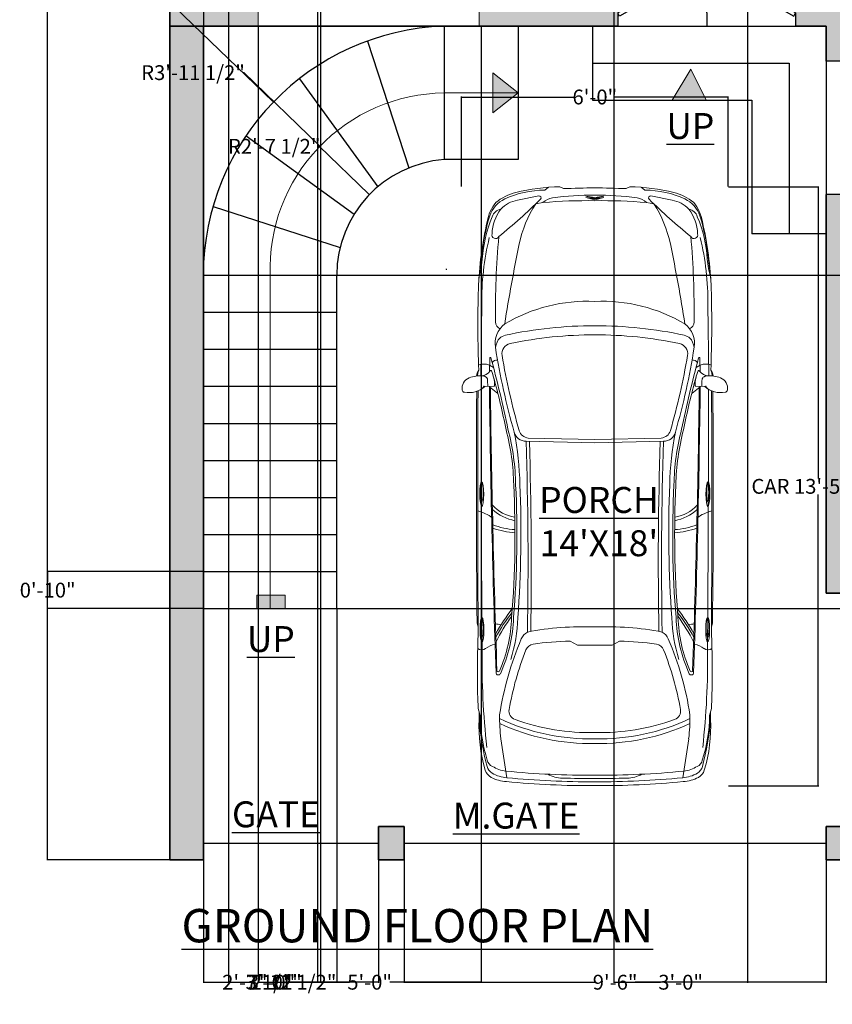
# Model space of a CAD drawing. Units: inches. Extents: x -37 to 408, y -619 to 75.
# Tile 1 of 4: x -37 to 182, y -619 to -354. Entities that reach past the tile are written whole.
import ezdxf

# ---------------------------------------------------------------- set-up
doc = ezdxf.new("R2010")
doc.units = ezdxf.units.IN
doc.header["$MEASUREMENT"] = 0
for name, color, linetype, lineweight in [('A-ANNO-DIMS', 2, 'Continuous', 18), ('A-ANNO-SYMB', 7, 'Continuous', 18), ('A-ANNO-TEXT', 7, 'Continuous', 25), ('A-AREA-IDEN', 7, 'Continuous', 25), ('A-DOOR', 4, 'Continuous', 25), ('A-FLOR-STRS', 7, 'Continuous', 25), ('A-GLAZ', 4, 'Continuous', 18), ('A-SITE-VEHI', 8, 'Continuous', 13), ('A-WALL', 7, 'Continuous', 35), ('A-WALL-PATT', 16, 'Continuous', 13)]:
    doc.layers.add(name, color=color, linetype=linetype, lineweight=lineweight)
doc.styles.get("Standard").update_dxf_attribs({"font": 'arial.ttf'})
doc.dimstyles.get("Standard").update_dxf_attribs({"dimtxt": 4, "dimasz": 0.18, "dimexe": 0.18, "dimexo": 0.0625, "dimgap": 0.09, "dimtad": 0, "dimtih": 1, "dimtoh": 1, "dimdec": 1, "dimzin": 0, "dimdsep": 46, "dimlunit": 4, "dimtxsty": 'Standard', "dimcen": 0.09, "dimadec": 0, "dimazin": 0, "dimtfac": 1, "dimtdec": 1, "dimtofl": 0, "dimtmove": 0, "dimatfit": 3, "dimfxl": 1, "dimtolj": 1, "dimtzin": 0, "dimarcsym": 0})

# ---------------------------------------------------------------- blocks, each defined once
blk = doc.blocks.new('*U2')
for p, q in [((0, 0), (0, -6)), ((40, 0), (40, -6))]:
    blk.add_line(p, q)
blk.add_lwpolyline([(0, 0), (34.64, 20), (35.52, 18.48), (0.87, -1.52)], close=True)
blk.add_arc((0, 0), 40, 0, 30)
blk = doc.blocks.new('A$C132F2E1D')
for p, q in [((0.543, 1.8886), (0.7013, 1.9079)), ((0.9043, 1.8866), (1.4518, 1.8937)), ((1.3706, 1.9103), (1.3631, 1.8926)), ((1.3631, 1.8926), (1.3631, 1.85)), ((1.407, 1.909), (1.4297, 1.9162)), ((1.4297, 1.9162), (1.4528, 1.9186)), ((3.3784, 1.9133), (3.3526, 1.9135)), ((3.3527, 1.9215), (3.3784, 1.9133)), ((3.3784, 1.9133), (3.5448, 1.9172)), ((4.008, 1.9136), (4.0609, 1.8993)), ((4.0895, 1.9062), (4.0345, 1.9064)), ((1.4203, 1.827), (1.3158, 1.8252)), ((1.3631, 1.85), (1.3696, 1.8261)), ((1.3696, 1.8261), (1.3875, 1.7961)), ((1.4882, 1.8409), (1.5335, 1.8395)), ((1.5342, 1.8622), (1.532, 1.7927)), ((1.5873, 1.7618), (1.5368, 1.8274)), ((2.5334, 1.8104), (2.5334, 1.8104)), ((4.24, 1.7387), (4.5389, 1.6933)), ((0.1023, 1.6121), (0.0698, 1.4487)), ((1.9298, 1.5286), (1.9419, 1.0174)), ((1.9544, 1.5457), (1.9669, 1.018)), ((0.12, 1.4158), (0.13, 1.4708)), ((0.0033, 1.3741), (0.0255, 1.4026)), ((0.0136, 1.2588), (0, 1.2857)), ((3.5213, 1.1507), (3.4897, 1.2072)), ((3.5213, 1.018), (3.5213, 1.1507)), ((0.0896, 1.018), (0.0719, 1.088)), ((0.0719, 1.088), (0.0821, 1.018)), ((0.1006, 1.018), (0.0828, 1.088)), ((0.0828, 1.088), (0.0931, 1.018)), ((0.0896, 1.018), (0.0719, 0.9479)), ((0.0719, 0.9479), (0.0821, 1.018)), ((0.1006, 1.018), (0.0828, 0.9479)), ((0.0828, 0.9479), (0.0931, 1.018)), ((1.9298, 0.5073), (1.9419, 1.0186)), ((1.9544, 0.4903), (1.9669, 1.018)), ((3.5213, 1.018), (3.5213, 0.8853)), ((3.5213, 0.8853), (3.4897, 0.8287)), ((0.0136, 0.7772), (0, 0.7503)), ((0.0033, 0.6619), (0.0255, 0.6334)), ((0.12, 0.6201), (0.13, 0.5651)), ((0.1023, 0.4239), (0.0698, 0.5873)), ((4.24, 0.2973), (4.5389, 0.3426)), ((1.3696, 0.2099), (1.3875, 0.2398)), ((1.5342, 0.1738), (1.532, 0.2432)), ((1.5873, 0.2742), (1.5368, 0.2086)), ((1.4203, 0.209), (1.3158, 0.2108)), ((1.3631, 0.186), (1.3696, 0.2099)), ((1.3631, 0.1434), (1.3631, 0.186)), ((1.4882, 0.1951), (1.5335, 0.1965)), ((2.5334, 0.2256), (2.5334, 0.2256)), ((0.543, 0.1473), (0.7013, 0.128)), ((0.9043, 0.1493), (1.4518, 0.1422)), ((1.3706, 0.1257), (1.3631, 0.1434)), ((1.407, 0.127), (1.4297, 0.1198)), ((1.4297, 0.1198), (1.4528, 0.1174)), ((3.3784, 0.1227), (3.3526, 0.1225)), ((3.3527, 0.1145), (3.3784, 0.1227)), ((3.3784, 0.1227), (3.5448, 0.1188)), ((4.008, 0.1224), (4.0609, 0.1367)), ((4.0895, 0.1298), (4.0345, 0.1295))]:
    blk.add_line(p, q)
for points in [[(0.5545, 1.882), (0.6265, 1.8906), (0.7013, 1.9079)], [(0.5545, 0.154), (0.6265, 0.1454), (0.7013, 0.128)]]:
    blk.add_lwpolyline(points)
for centre, radius, start, end in [((1.7253, 1.8951), 0.2735, 161.16843, 183.85292), ((1.5478, 1.9486), 0.0885, 81.04298, 156.83016), ((1.3899, 1.9873), 0.191, 319.07376, 9.749), ((1.5584, 2.0162), 0.02, 9.749, 81.04298), ((0.8722, -0.7564), 2.6698, 91.88228, 103.11637), ((1.0501, -7.5126), 9.4283, 87.83061, 91.61395), ((1.4598, 1.8405), 0.0865, 94.11262, 127.67305), ((1.357, 1.8976), 0.0949, 305.49305, 357.64193), ((1.1259, -373.2553), 375.1468, 89.629132, 89.934477), ((2.3981, -110.3129), 112.2304, 89.512732, 90.424576), ((2.3135, -85.6642), 87.5918, 89.32026, 90.486182), ((2.845, 2.0124), 0.3681, 194.95147, 214.73189), ((3.7262, -4.5417), 6.4614, 87.50012, 91.60876), ((3.5093, 1.8853), 0.0477, 322.74562, 41.97986), ((4.047, 0.7351), 1.1643, 72.17211, 89.31712), ((4.1487, 0.7567), 1.151, 73.23925, 92.94622), ((3.9598, 0.0566), 1.8542, 74.63039, 85.98685), ((0.2968, 1.612), 0.2258, 109.40449, 154.47293), ((0.3163, 1.539), 0.3088, 99.30607, 129.20262), ((0.7158, 0.1754), 1.7219, 95.75871, 106.66999), ((0.6164, 0.8965), 0.9874, 93.59221, 113.06049), ((0.8873, -0.259), 2.1457, 89.54661, 103.41209), ((1.3159, 1.8202), 0.005, 90.9623, 254.9067), ((3.6251, 10.2904), 8.7843, 254.74992, 258.42395), ((1.415, 1.8163), 0.005, 125.49305, 246.15831), ((1.4869, 1.8754), 0.0345, 177.75339, 272.27983), ((1.5189, 1.9076), 0.0394, 285.5168, 324.74311), ((0.383, -94.8685), 96.7028, 88.014877, 89.318555), ((0.383, -94.8685), 96.6953, 88.024999, 89.312887), ((3.6377, 1.7731), 0.1229, 137.35065, 175.10864), ((3.6347, -4.1374), 6.0215, 83.60515, 90.76636), ((4.3939, 1.7824), 0.0618, 20.2199, 81.07696), ((4.4332, 1.7639), 0.0825, 30.5014, 77.40713), ((4.4497, 1.7647), 0.0991, 29.59344, 71.79345), ((0.4002, 1.5413), 0.3661, 139.6653, 166.82313), ((-3.1006, 4.5928), 4.4926, 315.34452, 320.82807), ((0.3712, 1.4803), 0.3273, 91.86492, 127.65559), ((0.2504, 1.7277), 0.0801, 105.04002, 171.6116), ((0.3687, 1.7801), 0.0285, 298.61649, 106.64681), ((0.9479, -4.5143), 6.2948, 89.18041, 95.15468), ((1.0412, 1.7282), 0.0518, 20.25644, 93.59604), ((1.2013, 1.598), 0.1854, 80.28636, 142.92407), ((0.4389, -3.3422), 5.1841, 73.81498, 81.19317), ((1.3711, 1.7701), 0.0406, 119.08859, 187.71379), ((1.526, 2.0675), 0.2796, 246.15831, 270.21376), ((2.9375, 7.1081), 5.5139, 254.46339, 258.79798), ((1.527, 1.7929), 0.005, 270.21376, 358.17221), ((2.2304, 1.5809), 0.311, 9.49373, 46.03765), ((2.2118, 1.5633), 0.3589, 10.99766, 42.14068), ((1.9842, 1.583), 0.6504, 4.23296, 19.62219), ((1.8364, 1.5439), 0.8263, 6.04716, 18.12027), ((4.2291, 0.3611), 1.6261, 119.33405, 127.48815), ((3.9957, 0.7394), 1.168, 117.24964, 128.49508), ((4.1001, 0.5643), 1.3548, 116.50327, 126.3201), ((3.2695, 2.7758), 1.1198, 271.90334, 293.67172), ((3.2695, 2.7758), 1.1348, 271.90334, 294.46129), ((3.5501, 1.7951), 0.1937, 184.16269, 197.14768), ((4.4219, -0.6417), 2.4183, 98.71867, 113.11099), ((3.7151, 1.7594), 0.01, 293.67172, 88.025), ((3.7322, 1.7588), 0.0175, 294.46129, 88.01488), ((4.0772, 0.45), 1.2989, 82.79642, 90.96292), ((2.6323, 1.0566), 1.6082, 358.62448, 25.49807), ((2.6328, 1.0566), 1.6427, 358.62433, 24.89552), ((4.2402, 1.6718), 0.2494, 6.73694, 31.93348), ((4.2725, 1.6729), 0.2672, 4.38261, 29.81512), ((4.2692, 1.6755), 0.3003, 3.95205, 27.38435), ((0.7337, 1.4073), 0.7082, 154.75665, 180.37751), ((0.3282, 1.5721), 0.2294, 133.18069, 169.95622), ((3.0639, -11.0707), 12.9377, 98.94001, 101.70633), ((2.1201, 1.0748), 1.2415, 149.23442, 182.62114), ((4.2615, 1.0246), 3.195, 167.7045, 180.11803), ((4.2599, 1.0246), 3.1233, 168.11852, 180.1181), ((1.2818, 1.6513), 0.08, 80.41936, 168.20842), ((0.4389, -3.3422), 5.1441, 73.81498, 80.41936), ((2.3151, 3.3892), 1.7636, 255.12579, 269.16493), ((2.3151, 3.3892), 1.7486, 255.12579, 269.16493), ((4.4219, -0.6417), 2.3533, 99.98189, 111.58148), ((4.0261, 1.6071), 0.07, 19.45244, 99.98189), ((-2.0942, 1.0548), 6.6138, 359.68361, 5.60781), ((-2.0924, 1.0548), 6.662, 359.68358, 5.50038), ((-2.0924, 1.0548), 6.692, 359.68359, 5.5002), ((1.3941, 1.2785), 1.3941, 165.61673, 179.7063), ((0.615, 0.7306), 0.885, 101.47468, 123.23035), ((1.8484, 1.5199), 0.0818, 6.1177, 72.66243), ((2.3534, 4.0946), 2.5026, 259.18744, 268.48682), ((1.861, 1.5459), 0.0934, 359.82686, 75.78413), ((2.6538, 10.9506), 9.3649, 267.75715, 274.02026), ((2.6795, 9.2996), 7.6836, 267.08589, 274.69152), ((2.6795, 9.2996), 7.6686, 267.08589, 274.69152), ((3.2609, 2.8713), 1.2635, 272.24484, 286.98853), ((2.4672, 1.0516), 1.7249, 358.88416, 19.60736), ((2.8877, 30.3882), 28.8577, 268.14656, 271.05631), ((2.8877, 30.3882), 28.8827, 268.14933, 271.04617), ((5.6577, 1.1038), 2.2792, 169.08169, 182.15619), ((3.5126, 1.4843), 0.106, 112.12502, 151.18035), ((3.582, 1.4816), 0.07, 111.58148, 171.48298), ((0.0845, 1.4458), 0.015, 168.75011, 315.34452), ((5.6068, 1.1784), 2.1173, 171.48298, 179.21912), ((0.2091, 1.3272), 0.1256, 135.16316, 173.03669), ((4.4703, 1.065), 4.3644, 175.38888, 180.61666), ((4.3309, 1.2705), 0.2103, 358.93016, 30.75657), ((2.4077, 1.0327), 2.3439, 172.40644, 180.3604), ((-18.6368, 1.714), 18.656, 357.86205, 358.60201), ((-1.9281, 1.0543), 6.4726, 359.67956, 1.87886), ((-18.6368, 0.322), 18.656, 1.39799, 2.13795), ((2.4077, 1.0032), 2.3439, 179.6396, 187.59356), ((4.4703, 0.971), 4.3644, 179.38334, 184.61112), ((2.1201, 0.9612), 1.2415, 177.37886, 210.76558), ((4.2615, 1.0114), 3.195, 179.88197, 192.2955), ((4.2599, 1.0114), 3.1233, 179.8819, 191.88148), ((5.6577, 0.9322), 2.2792, 177.84381, 190.91831), ((2.6323, 0.9794), 1.6082, 334.50193, 1.37552), ((2.4672, 0.9844), 1.7249, 340.39264, 1.11584), ((2.6328, 0.9794), 1.6427, 335.10448, 1.37567), ((-2.0942, 0.9812), 6.6138, 354.39219, 0.31639), ((-2.0924, 0.9812), 6.662, 354.49962, 0.31642), ((-1.9281, 0.9816), 6.4726, 358.12114, 0.32044), ((-2.0924, 0.9812), 6.692, 354.4998, 0.31641), ((5.6068, 0.8576), 2.1173, 180.78088, 188.51702), ((4.3309, 0.7655), 0.2103, 329.24343, 1.06984), ((1.3941, 0.7575), 1.3941, 180.2937, 194.38327), ((0.2091, 0.7087), 0.1256, 186.96331, 224.83684), ((0.7337, 0.6287), 0.7082, 179.62249, 205.24335), ((0.0845, 0.5902), 0.015, 44.65548, 191.24989), ((-3.1006, -2.5569), 4.4926, 39.17193, 44.65548), ((0.615, 1.3054), 0.885, 236.76965, 258.52532), ((2.8877, -28.3523), 28.8827, 88.95383, 91.85067), ((3.582, 0.5544), 0.07, 188.51702, 248.41852), ((1.8484, 0.516), 0.0818, 287.33757, 353.8823), ((1.861, 0.49), 0.0934, 284.21587, 0.17314), ((2.8877, -28.3523), 28.8577, 88.94369, 91.85344), ((3.5126, 0.5516), 0.106, 208.81965, 247.87498), ((4.4219, 2.6776), 2.3533, 248.41852, 260.01811), ((0.4002, 0.4946), 0.3661, 193.17687, 220.3347), ((0.3282, 0.4639), 0.2294, 190.04378, 226.81931), ((3.0639, 13.1067), 12.9377, 258.29367, 261.05999), ((0.4389, 5.3782), 5.1841, 278.80683, 286.18502), ((0.4389, 5.3782), 5.1441, 279.58064, 286.18502), ((2.3151, -1.3533), 1.7636, 90.83507, 104.87421), ((2.3151, -1.3533), 1.7486, 90.83507, 104.87421), ((2.3534, -2.0587), 2.5026, 91.51318, 100.81256), ((2.6538, -8.9146), 9.3649, 85.97974, 92.24285), ((2.6795, -7.2636), 7.6836, 85.30848, 92.91411), ((2.6795, -7.2636), 7.6686, 85.30848, 92.91411), ((2.2304, 0.455), 0.311, 313.96235, 350.50627), ((2.2118, 0.4726), 0.3589, 317.85932, 349.00234), ((1.9842, 0.4529), 0.6504, 340.37781, 355.76704), ((1.8364, 0.4921), 0.8263, 341.87973, 353.95284), ((4.2291, 1.6749), 1.6261, 232.51185, 240.66595), ((3.9957, 1.2965), 1.168, 231.50492, 242.75036), ((4.1001, 1.4717), 1.3548, 233.6799, 243.49673), ((3.2695, -0.7398), 1.1198, 66.32828, 88.09666), ((3.2695, -0.7398), 1.1348, 65.53871, 88.09666), ((3.2609, -0.8353), 1.2635, 73.01147, 87.75516), ((4.4219, 2.6776), 2.4183, 246.88901, 261.28133), ((4.0261, 0.4289), 0.07, 260.01811, 340.54756), ((0.2968, 0.424), 0.2258, 205.52707, 250.59551), ((1.2013, 0.438), 0.1854, 217.07593, 279.71364), ((1.2818, 0.3847), 0.08, 191.79158, 279.58064), ((3.6251, -8.2544), 8.7843, 101.57605, 105.25008), ((2.9375, -5.0721), 5.5139, 101.20202, 105.53661), ((4.2402, 0.3642), 0.2494, 328.06652, 353.26306), ((4.2725, 0.363), 0.2672, 330.18488, 355.61739), ((4.2692, 0.3605), 0.3003, 332.61565, 356.04795), ((0.3163, 0.497), 0.3088, 230.79738, 260.69393), ((0.3712, 0.5557), 0.3273, 232.34441, 268.13508), ((0.2504, 0.3083), 0.0801, 188.3884, 254.95998), ((0.6164, 1.1394), 0.9874, 246.93951, 266.40779), ((0.3687, 0.2559), 0.0285, 253.35319, 61.38351), ((0.9479, 6.5502), 6.2948, 264.84532, 270.81959), ((1.0412, 0.3078), 0.0518, 266.40396, 339.74356), ((1.3711, 0.2659), 0.0406, 172.28621, 240.91141), ((1.526, -0.0316), 0.2796, 89.78624, 113.84169), ((1.527, 0.2431), 0.005, 1.82779, 89.78624), ((0.383, 96.9045), 96.7028, 270.681445, 271.985123), ((0.383, 96.9045), 96.6953, 270.687113, 271.975001), ((2.845, 0.0236), 0.3681, 145.26811, 165.04853), ((3.5501, 0.2409), 0.1937, 162.85232, 175.83731), ((3.6377, 0.2629), 0.1229, 184.89136, 222.64935), ((3.7151, 0.2766), 0.01, 271.975, 66.32828), ((3.7322, 0.2772), 0.0175, 271.98512, 65.53871), ((4.0772, 1.5859), 1.2989, 269.03708, 277.20358), ((4.3939, 0.2536), 0.0618, 278.92304, 339.7801), ((4.4332, 0.2721), 0.0825, 282.59287, 329.4986), ((0.7158, 1.8606), 1.7219, 253.33001, 264.24129), ((0.8722, 2.7923), 2.6698, 256.88363, 268.11772), ((0.8873, 2.295), 2.1457, 256.58791, 270.45339), ((1.3159, 0.2158), 0.005, 105.0933, 269.0377), ((1.415, 0.2196), 0.005, 113.84169, 234.50695), ((1.357, 0.1383), 0.0949, 2.35807, 54.50695), ((1.7253, 0.1409), 0.2735, 176.14708, 198.83157), ((1.4869, 0.1606), 0.0345, 87.72017, 182.24661), ((1.5189, 0.1283), 0.0394, 35.25689, 74.4832), ((1.3899, 0.0487), 0.191, 350.251, 40.92624), ((1.1259, 375.2913), 375.1468, 270.065523, 270.370868), ((3.5093, 0.1507), 0.0477, 318.02014, 37.25438), ((3.6347, 6.1734), 6.0215, 269.23364, 276.39485), ((4.047, 1.3009), 1.1643, 270.68288, 287.82789), ((3.9598, 1.9794), 1.8542, 274.01315, 285.36961), ((4.1487, 1.2793), 1.151, 267.05378, 286.76075), ((4.4497, 0.2713), 0.0991, 288.20655, 330.40656), ((1.0501, 9.5485), 9.4283, 268.38605, 272.16939), ((1.4598, 0.1954), 0.0865, 232.32695, 265.88738), ((2.3981, 112.3489), 112.2304, 269.575424, 270.487268), ((2.3135, 87.7001), 87.5918, 269.513818, 270.67974), ((3.7262, 6.5777), 6.4614, 268.39124, 272.49988), ((1.5478, 0.0874), 0.0885, 203.16984, 278.95702), ((1.5584, 0.0197), 0.02, 278.95702, 350.251)]:
    blk.add_arc(centre, radius, start, end)
for centre, major_axis in [((2.3605, 1.8864), (0.0938, -0.0005)), ((2.3473, 1.8864), (0.0703, -0.0004)), ((3.401, 1.8845), (0.0938, -0.0005)), ((3.3878, 1.8845), (0.0703, -0.0004))]:
    blk.add_ellipse(centre, major_axis=major_axis, ratio=0.16097)
at = {"extrusion": (0, 0, -1)}
for centre, major_axis in [((2.3605, 0.1496), (0.0938, 0.0005)), ((2.3473, 0.1495), (0.0703, 0.0004)), ((3.401, 0.1515), (0.0938, 0.0005)), ((3.3878, 0.1514), (0.0703, 0.0004))]:
    blk.add_ellipse(centre, major_axis=major_axis, ratio=0.16097, dxfattribs=at)
for points in [[(1.1398, 1.7049), (1.1459, 1.7208), (1.1615, 1.7621), (1.2055, 1.7737), (1.2326, 1.7808)], [(1.1398, 0.331), (1.1459, 0.3151), (1.1615, 0.2739), (1.2055, 0.2623), (1.2326, 0.2552)]]:
    blk.add_open_spline(points, degree=3, knots=[0, 0, 0, 0, 0.0487, 0.1263518, 0.1263518, 0.1263518, 0.1263518])
blk = doc.blocks.new('*D24')
at = {"layer": 'A-ANNO-DIMS', "color": 0, "lineweight": -2, "transparency": 16777216}
for p, q in [((154.24, -398.74), (178.6, -398.74)), ((178.42, -398.92), (178.42, -477.4)), ((178.42, -560.19), (178.42, -481.72)), ((154.24, -560.37), (178.6, -560.37))]:
    blk.add_line(p, q, dxfattribs=at)
at = {"layer": 'A-ANNO-DIMS', "color": 0, "transparency": 16777216}
for points in [[(178.39, -398.92), (178.45, -398.92), (178.42, -398.74)], [(178.39, -560.19), (178.45, -560.19), (178.42, -560.37)]]:
    blk.add_solid(points, dxfattribs=at)
at = {"layer": 'Defpoints', "color": 0, "transparency": 16777216}
for p in [(154.18, -398.74), (154.18, -560.37), (178.42, -560.37)]:
    blk.add_point(p, dxfattribs=at)
at = {"layer": 'A-ANNO-DIMS', "color": 0, "transparency": 16777216, "insert": (178.42, -479.56), "char_height": 4, "attachment_point": 5}
blk.add_mtext('\\A1;CAR 13\'-5 1/2"', dxfattribs=at)
blk = doc.blocks.new('*D25')
at = {"layer": 'A-ANNO-DIMS', "color": 0, "lineweight": -2, "transparency": 16777216}
for p, q in [((82.2, -398.68), (82.2, -374.31)), ((82.38, -374.49), (112.77, -374.49)), ((154, -374.49), (123.61, -374.49)), ((154.18, -398.68), (154.18, -374.31))]:
    blk.add_line(p, q, dxfattribs=at)
at = {"layer": 'A-ANNO-DIMS', "color": 0, "transparency": 16777216}
for points in [[(82.38, -374.46), (82.38, -374.52), (82.2, -374.49)], [(154, -374.46), (154, -374.52), (154.18, -374.49)]]:
    blk.add_solid(points, dxfattribs=at)
at = {"layer": 'Defpoints', "color": 0, "transparency": 16777216}
for p in [(154.18, -374.49), (82.2, -398.74), (154.18, -398.74)]:
    blk.add_point(p, dxfattribs=at)
at = {"layer": 'A-ANNO-DIMS', "color": 0, "transparency": 16777216, "insert": (118.19, -374.49), "char_height": 4, "attachment_point": 5}
blk.add_mtext('\\A1;6\'-0"', dxfattribs=at)
blk = doc.blocks.new('*D28')
at = {"layer": 'A-ANNO-DIMS', "color": 0, "lineweight": -2, "transparency": 16777216}
for p, q in [((3.52, 28.62), (-29.6, 28.62)), ((-29.42, 28.44), (-29.42, -273.74)), ((-29.42, -580.2), (-29.42, -278.01)), ((3.52, -580.38), (-29.6, -580.38))]:
    blk.add_line(p, q, dxfattribs=at)
at = {"layer": 'A-ANNO-DIMS', "color": 0, "transparency": 16777216}
for points in [[(-29.45, 28.44), (-29.39, 28.44), (-29.42, 28.62)], [(-29.45, -580.2), (-29.39, -580.2), (-29.42, -580.38)]]:
    blk.add_solid(points, dxfattribs=at)
at = {"layer": 'Defpoints', "color": 0, "transparency": 16777216}
for p in [(-29.42, 28.62), (3.58, 28.62), (3.58, -580.38)]:
    blk.add_point(p, dxfattribs=at)
at = {"layer": 'A-ANNO-DIMS', "color": 0, "transparency": 16777216, "insert": (-29.42, -275.88), "char_height": 4, "attachment_point": 5}
blk.add_mtext('\\A1;50\'-9"', dxfattribs=at)
blk = doc.blocks.new('*D30')
at = {"layer": 'A-ANNO-DIMS', "color": 0, "lineweight": -2, "transparency": 16777216}
for p, q in [((12.58, -512.63), (12.58, -613.56)), ((48.58, -512.63), (48.58, -613.56)), ((12.76, -613.38), (25.17, -613.38)), ((48.4, -613.38), (35.98, -613.38))]:
    blk.add_line(p, q, dxfattribs=at)
at = {"layer": 'A-ANNO-DIMS', "color": 0, "transparency": 16777216}
for points in [[(12.76, -613.35), (12.76, -613.41), (12.58, -613.38)], [(48.4, -613.35), (48.4, -613.41), (48.58, -613.38)]]:
    blk.add_solid(points, dxfattribs=at)
at = {"layer": 'Defpoints', "color": 0, "transparency": 16777216}
for p in [(12.58, -512.57), (48.58, -512.57), (48.58, -613.38)]:
    blk.add_point(p, dxfattribs=at)
at = {"layer": 'A-ANNO-DIMS', "color": 0, "transparency": 16777216, "insert": (30.58, -613.38), "char_height": 4, "attachment_point": 5}
blk.add_mtext('\\A1;3\'-0"', dxfattribs=at)
blk = doc.blocks.new('*D32')
at = {"layer": 'A-ANNO-DIMS', "color": 0, "lineweight": -2, "transparency": 16777216}
for p, q in [((12.58, -580.44), (12.58, -613.56)), ((59.87, -580.44), (59.87, -613.56)), ((12.76, -613.38), (24.6, -613.38)), ((59.69, -613.38), (47.84, -613.38))]:
    blk.add_line(p, q, dxfattribs=at)
at = {"layer": 'A-ANNO-DIMS', "color": 0, "transparency": 16777216}
for points in [[(12.76, -613.35), (12.76, -613.41), (12.58, -613.38)], [(59.69, -613.35), (59.69, -613.41), (59.87, -613.38)]]:
    blk.add_solid(points, dxfattribs=at)
at = {"layer": 'Defpoints', "color": 0, "transparency": 16777216}
for p in [(12.58, -580.38), (59.87, -580.38), (59.87, -613.38)]:
    blk.add_point(p, dxfattribs=at)
at = {"layer": 'A-ANNO-DIMS', "color": 0, "transparency": 16777216, "insert": (36.22, -613.38), "char_height": 4, "attachment_point": 5}
blk.add_mtext('\\A1;3\'-11 1/2"', dxfattribs=at)
blk = doc.blocks.new('*D33')
at = {"layer": 'A-ANNO-DIMS', "color": 0, "lineweight": -2, "transparency": 16777216}
for p, q in [((66.73, -580.44), (66.73, -613.56)), ((180.58, -580.44), (180.58, -613.56)), ((66.91, -613.38), (118.25, -613.38)), ((180.4, -613.38), (129.06, -613.38))]:
    blk.add_line(p, q, dxfattribs=at)
at = {"layer": 'A-ANNO-DIMS', "color": 0, "transparency": 16777216}
for points in [[(66.91, -613.35), (66.91, -613.41), (66.73, -613.38)], [(180.4, -613.35), (180.4, -613.41), (180.58, -613.38)]]:
    blk.add_solid(points, dxfattribs=at)
at = {"layer": 'Defpoints', "color": 0, "transparency": 16777216}
for p in [(66.73, -580.38), (180.58, -580.38), (180.58, -613.38)]:
    blk.add_point(p, dxfattribs=at)
at = {"layer": 'A-ANNO-DIMS', "color": 0, "transparency": 16777216, "insert": (123.66, -613.38), "char_height": 4, "attachment_point": 5}
blk.add_mtext('\\A1;9\'-6"', dxfattribs=at)
blk = doc.blocks.new('*D36')
at = {"layer": 'A-ANNO-DIMS', "color": 0, "lineweight": -2, "transparency": 16777216}
for p, q in [((27.35, -355.44), (27.35, -613.56)), ((87.53, -355.44), (87.53, -613.56)), ((27.53, -613.38), (52.03, -613.38)), ((87.35, -613.38), (62.85, -613.38))]:
    blk.add_line(p, q, dxfattribs=at)
at = {"layer": 'A-ANNO-DIMS', "color": 0, "transparency": 16777216}
for points in [[(27.53, -613.35), (27.53, -613.41), (27.35, -613.38)], [(87.35, -613.35), (87.35, -613.41), (87.53, -613.38)]]:
    blk.add_solid(points, dxfattribs=at)
at = {"layer": 'Defpoints', "color": 0, "transparency": 16777216}
for p in [(27.35, -355.38), (87.53, -355.38), (87.53, -613.38)]:
    blk.add_point(p, dxfattribs=at)
at = {"layer": 'A-ANNO-DIMS', "color": 0, "transparency": 16777216, "insert": (57.44, -613.38), "char_height": 4, "attachment_point": 5}
blk.add_mtext('\\A1;5\'-0"', dxfattribs=at)
blk = doc.blocks.new('*D37')
at = {"layer": 'A-ANNO-DIMS', "color": 0, "lineweight": -2, "transparency": 16777216}
for p, q in [((12.58, -214.44), (12.58, -613.56)), ((44.21, -214.44), (44.21, -613.56)), ((12.76, -613.38), (18.3, -613.38)), ((44.03, -613.38), (38.5, -613.38))]:
    blk.add_line(p, q, dxfattribs=at)
at = {"layer": 'A-ANNO-DIMS', "color": 0, "transparency": 16777216}
for points in [[(12.76, -613.35), (12.76, -613.41), (12.58, -613.38)], [(44.03, -613.35), (44.03, -613.41), (44.21, -613.38)]]:
    blk.add_solid(points, dxfattribs=at)
at = {"layer": 'Defpoints', "color": 0, "transparency": 16777216}
for p in [(12.58, -214.38), (44.21, -214.38), (44.21, -613.38)]:
    blk.add_point(p, dxfattribs=at)
at = {"layer": 'A-ANNO-DIMS', "color": 0, "transparency": 16777216, "insert": (28.4, -613.38), "char_height": 4, "attachment_point": 5}
blk.add_mtext('\\A1;2\'-7 1/2"', dxfattribs=at)
blk = doc.blocks.new('*D38')
at = {"layer": 'A-ANNO-DIMS', "color": 0, "lineweight": -2, "transparency": 16777216}
for p, q in [((123.34, -214.44), (123.34, -613.56)), ((159.34, -214.44), (159.34, -613.56)), ((123.52, -613.38), (135.93, -613.38)), ((159.16, -613.38), (146.74, -613.38))]:
    blk.add_line(p, q, dxfattribs=at)
at = {"layer": 'A-ANNO-DIMS', "color": 0, "transparency": 16777216}
for points in [[(123.52, -613.35), (123.52, -613.41), (123.34, -613.38)], [(159.16, -613.35), (159.16, -613.41), (159.34, -613.38)]]:
    blk.add_solid(points, dxfattribs=at)
at = {"layer": 'Defpoints', "color": 0, "transparency": 16777216}
for p in [(123.34, -214.38), (159.34, -214.38), (159.34, -613.38)]:
    blk.add_point(p, dxfattribs=at)
at = {"layer": 'A-ANNO-DIMS', "color": 0, "transparency": 16777216, "insert": (141.34, -613.38), "char_height": 4, "attachment_point": 5}
blk.add_mtext('\\A1;3\'-0"', dxfattribs=at)
blk = doc.blocks.new('*D39')
at = {"layer": 'A-ANNO-DIMS', "color": 0, "lineweight": -2, "transparency": 16777216}
for p, q in [((19.34, -49.44), (19.34, -613.56)), ((43.34, -49.44), (43.34, -613.56)), ((19.52, -613.38), (25.9, -613.38)), ((43.16, -613.38), (36.78, -613.38))]:
    blk.add_line(p, q, dxfattribs=at)
at = {"layer": 'A-ANNO-DIMS', "color": 0, "transparency": 16777216}
for points in [[(19.52, -613.35), (19.52, -613.41), (19.34, -613.38)], [(43.16, -613.35), (43.16, -613.41), (43.34, -613.38)]]:
    blk.add_solid(points, dxfattribs=at)
at = {"layer": 'Defpoints', "color": 0, "transparency": 16777216}
for p in [(19.34, -49.38), (43.34, -49.38), (43.34, -613.38)]:
    blk.add_point(p, dxfattribs=at)
at = {"layer": 'A-ANNO-DIMS', "color": 0, "transparency": 16777216, "insert": (31.34, -613.38), "char_height": 4, "attachment_point": 5}
blk.add_mtext('\\A1;2\'-0"', dxfattribs=at)
blk = doc.blocks.new('*D41')
at = {"layer": 'A-ANNO-DIMS', "color": 0, "lineweight": -2, "transparency": 16777216}
for p, q in [((12.52, -502.57), (-29.6, -502.57)), ((-29.42, -502.75), (-29.42, -505.43)), ((-29.42, -512.39), (-29.42, -509.7)), ((12.52, -512.57), (-29.6, -512.57))]:
    blk.add_line(p, q, dxfattribs=at)
at = {"layer": 'A-ANNO-DIMS', "color": 0, "transparency": 16777216}
for points in [[(-29.45, -502.75), (-29.39, -502.75), (-29.42, -502.57)], [(-29.45, -512.39), (-29.39, -512.39), (-29.42, -512.57)]]:
    blk.add_solid(points, dxfattribs=at)
at = {"layer": 'Defpoints', "color": 0, "transparency": 16777216}
for p in [(-29.42, -502.57), (12.58, -502.57), (12.58, -512.57)]:
    blk.add_point(p, dxfattribs=at)
at = {"layer": 'A-ANNO-DIMS', "color": 0, "transparency": 16777216, "insert": (-29.42, -507.57), "char_height": 4, "attachment_point": 5}
blk.add_mtext('\\A1;0\'-10"', dxfattribs=at)
blk = doc.blocks.new('*D42')
at = {"layer": 'A-ANNO-DIMS', "color": 0, "lineweight": -2, "transparency": 16777216}
for p, q in [((48.64, -422.57), (396.76, -422.57)), ((396.58, -422.75), (396.58, -465.43)), ((396.58, -512.39), (396.58, -469.7)), ((48.64, -512.57), (396.76, -512.57))]:
    blk.add_line(p, q, dxfattribs=at)
at = {"layer": 'A-ANNO-DIMS', "color": 0, "transparency": 16777216}
for points in [[(396.55, -422.75), (396.61, -422.75), (396.58, -422.57)], [(396.55, -512.39), (396.61, -512.39), (396.58, -512.57)]]:
    blk.add_solid(points, dxfattribs=at)
at = {"layer": 'Defpoints', "color": 0, "transparency": 16777216}
for p in [(48.58, -422.57), (396.58, -422.57), (48.58, -512.57)]:
    blk.add_point(p, dxfattribs=at)
at = {"layer": 'A-ANNO-DIMS', "color": 0, "transparency": 16777216, "insert": (396.58, -467.57), "char_height": 4, "attachment_point": 5}
blk.add_mtext('\\A1;7\'-6"', dxfattribs=at)
blk = doc.blocks.new('*D54')
at = {"layer": 'A-ANNO-DIMS', "color": 0, "lineweight": -2, "transparency": 16777216}
for p, q in [((2.29, -347.81), (2.47, -347.81)), ((2.47, -347.81), (31.34, -375.72)), ((79.81, -422.66), (79.81, -422.48)), ((79.72, -422.57), (79.9, -422.57))]:
    blk.add_line(p, q, dxfattribs=at)
at = {"layer": 'A-ANNO-DIMS', "color": 0, "transparency": 16777216}
blk.add_solid([(31.36, -375.7), (31.32, -375.74), (31.47, -375.84)], dxfattribs=at)
at = {"layer": 'Defpoints', "color": 0, "transparency": 16777216}
for p in [(31.47, -375.84), (79.81, -422.57)]:
    blk.add_point(p, dxfattribs=at)
at = {"layer": 'A-ANNO-DIMS', "color": 0, "transparency": 16777216, "insert": (-5.03, -347.81), "char_height": 4, "attachment_point": 5}
blk.add_mtext('\\A1;R5\'-7"', dxfattribs=at)
blk = doc.blocks.new('*D55')
at = {"layer": 'A-ANNO-DIMS', "color": 0, "lineweight": -2, "transparency": 16777216}
for p, q in [((43.68, -387.8), (43.86, -387.8)), ((43.86, -387.8), (57.23, -400.72)), ((79.85, -422.66), (79.85, -422.48)), ((79.76, -422.57), (79.94, -422.57))]:
    blk.add_line(p, q, dxfattribs=at)
at = {"layer": 'A-ANNO-DIMS', "color": 0, "transparency": 16777216}
blk.add_solid([(57.25, -400.69), (57.21, -400.74), (57.36, -400.84)], dxfattribs=at)
at = {"layer": 'Defpoints', "color": 0, "transparency": 16777216}
for p in [(57.36, -400.84), (79.85, -422.57)]:
    blk.add_point(p, dxfattribs=at)
at = {"layer": 'A-ANNO-DIMS', "color": 0, "transparency": 16777216, "insert": (31.7, -387.8), "char_height": 4, "attachment_point": 5}
blk.add_mtext('\\A1;R2\'-7 1/2"', dxfattribs=at)
blk = doc.blocks.new('*D56')
at = {"layer": 'A-ANNO-DIMS', "color": 0, "lineweight": -2, "transparency": 16777216}
for p, q in [((23.33, -367.92), (23.51, -367.92)), ((23.51, -367.92), (43.87, -387.68)), ((78.05, -420.96), (78.23, -420.96)), ((78.14, -421.05), (78.14, -420.87))]:
    blk.add_line(p, q, dxfattribs=at)
at = {"layer": 'A-ANNO-DIMS', "color": 0, "transparency": 16777216}
blk.add_solid([(43.89, -387.66), (43.85, -387.7), (44, -387.81)], dxfattribs=at)
at = {"layer": 'Defpoints', "color": 0, "transparency": 16777216}
for p in [(44, -387.81), (78.14, -420.96)]:
    blk.add_point(p, dxfattribs=at)
at = {"layer": 'A-ANNO-DIMS', "color": 0, "transparency": 16777216, "insert": (9.8, -367.92), "char_height": 4, "attachment_point": 5}
blk.add_mtext('\\A1;R3\'-11 1/2"', dxfattribs=at)

msp = doc.modelspace()

# ---------------------------------------------------------------- hatches: boundary and pattern name
at = {"layer": 'A-ANNO-SYMB'}
h = msp.add_hatch(color=256, dxfattribs=at)
h.dxf.hatch_style = 1
h.paths.add_polyline_path([(90.67, -367.98), (90.67, -373.38), (97.53, -373.38)])
h.paths.add_polyline_path([(97.53, -373.38), (90.67, -373.38), (90.67, -378.78)])
h = msp.add_hatch(color=256, dxfattribs=at)
h.dxf.hatch_style = 1
h.paths.add_polyline_path([(144.12, -367), (139.08, -375.38), (148.2, -375.38)])
h = msp.add_hatch(color=256, dxfattribs=at)
h.dxf.hatch_style = 1
h.paths.add_polyline_path([(30.58, -508.94), (27, -508.94), (27, -512.57), (30.58, -512.57)])
h.paths.add_polyline_path([(34.65, -508.94), (30.58, -508.94), (30.58, -512.57), (34.65, -512.57)])
at = {"layer": 'A-WALL-PATT'}
h = msp.add_hatch(color=256, dxfattribs=at)
h.dxf.hatch_style = 1
h.paths.add_polyline_path([(123.52, -205.38), (3.58, -205.38), (3.58, -355.38), (27.35, -355.38), (27.35, -346.38), (12.58, -346.38), (12.58, -214.38), (123.34, -214.38), (123.34, -208.98, -0.025047)])
h.paths.add_polyline_path([(117.58, -214.38), (108.58, -214.38), (108.58, -221.31), (112.18, -221.31), (117.58, -221.31)], flags=17)
h.paths.add_polyline_path([(124.36, -346.38), (86.98, -346.38), (86.98, -355.38), (124.36, -355.38), (124.36, -351.78)])
h.paths.add_polyline_path([(222.97, -346.38), (172.36, -346.38), (172.36, -351.78), (172.36, -355.38), (180.58, -355.38), (180.58, -364.83), (185.98, -364.83), (189.58, -364.83), (189.58, -355.38), (222.97, -355.38)])
h.paths.add_polyline_path([(363.58, -205.38), (241.29, -205.38, -0.025047), (241.47, -208.98), (241.47, -214.38), (354.58, -214.38), (354.58, -346.38), (317.68, -346.38), (317.68, -355.38), (363.58, -355.38)])
h = msp.add_hatch(color=256, dxfattribs=at)
h.dxf.hatch_style = 1
h.paths.add_polyline_path([(363.58, -355.38), (354.58, -355.38), (354.58, -499.38), (349.43, -499.38), (349.43, -502.98), (349.43, -508.38), (354.58, -508.38), (354.58, -571.38), (324.75, -571.38), (324.75, -580.38), (363.58, -580.38)])
h.paths.add_polyline_path([(291.68, -571.38), (261.58, -571.38), (261.58, -580.38), (291.68, -580.38)])
h.paths.add_polyline_path([(270.58, -508.38), (261.58, -508.38), (261.58, -571.38), (270.58, -571.38)])
h.paths.add_polyline_path([(325.43, -499.38), (258.03, -499.38), (258.03, -508.38), (326.04, -508.38, -0.056797), (325.43, -502.98)])
h.paths.add_polyline_path([(189.58, -571.38), (180.58, -571.38), (180.58, -580.38), (189.58, -580.38)])
h.paths.add_polyline_path([(189.58, -400.65, -0.025047), (185.98, -400.83), (180.58, -400.83), (180.58, -508.38), (189.58, -508.38), (197.89, -508.38), (197.89, -499.38), (189.58, -499.38)])
h.paths.add_polyline_path([(66.73, -571.38), (59.87, -571.38), (59.87, -580.38), (66.73, -580.38)])
h.paths.add_polyline_path([(12.58, -355.38), (3.58, -355.38), (3.58, -580.38), (12.58, -580.38), (12.58, -571.38)])

# ---------------------------------------------------------------- linework, layer by layer
at = {"layer": 'A-ANNO-SYMB'}
for p, q in [((97.53, -373.38), (90.67, -367.98)), ((90.67, -367.98), (90.67, -373.38)), ((139.08, -375.38), (144.12, -367)), ((144.12, -367), (148.2, -375.38)), ((97.53, -373.38), (77.53, -373.38)), ((97.53, -373.38), (90.67, -378.78)), ((90.67, -378.78), (90.67, -373.38)), ((30.58, -512.57), (30.58, -422.57)), ((27, -512.57), (27, -508.94)), ((27, -508.94), (34.65, -508.94)), ((34.65, -508.94), (34.65, -512.57))]:
    msp.add_line(p, q, dxfattribs=at)
msp.add_arc((78.14, -420.96), 47.58, 90.7343, 181.9385, dxfattribs=at)
at = {"layer": 'A-DOOR'}
for p, q in [((124.36, -355.38), (172.36, -355.38)), ((180.58, -364.83), (180.58, -400.83)), ((12.58, -575.88), (59.87, -575.88)), ((66.73, -575.88), (180.58, -575.88))]:
    msp.add_line(p, q, dxfattribs=at)
at = {"layer": 'A-FLOR-STRS'}
for p, q in [((77.53, -355.38), (77.53, -391.38)), ((87.53, -355.38), (87.53, -391.38)), ((97.53, -355.38), (97.53, -391.38)), ((117.58, -355.38), (117.58, -375.38)), ((56.88, -359.38), (68, -393.62)), ((117.58, -365.38), (170.58, -365.38)), ((170.58, -365.38), (170.58, -411.4)), ((38.48, -369.58), (59.64, -398.7)), ((117.58, -375.38), (160.58, -375.38)), ((160.58, -375.38), (160.58, -411.4)), ((24.13, -384.96), (53.25, -406.12)), ((97.53, -391.38), (77.53, -391.38)), ((15.23, -404.02), (49.47, -415.14)), ((180.58, -411.4), (160.58, -411.4)), ((12.58, -422.57), (48.58, -422.57)), ((48.58, -512.57), (48.58, -422.57)), ((12.58, -432.57), (48.58, -432.57)), ((12.58, -442.57), (48.58, -442.57)), ((12.58, -452.57), (48.58, -452.57)), ((12.58, -462.57), (48.58, -462.57)), ((12.58, -472.57), (48.58, -472.57)), ((12.58, -482.57), (48.58, -482.57)), ((12.58, -492.57), (48.58, -492.57)), ((12.58, -502.57), (48.58, -502.57)), ((12.58, -512.57), (48.58, -512.57))]:
    msp.add_line(p, q, dxfattribs=at)
for centre, radius, start in [((79.81, -422.57), 67.23, 91.9448), ((79.85, -422.57), 31.28, 94.2717)]:
    msp.add_arc(centre, radius, start, 180, dxfattribs=at)
at = {"layer": 'A-GLAZ'}
for p, q in [((27.35, -346.38), (27.35, -355.38)), ((86.98, -346.38), (86.98, -355.38))]:
    msp.add_line(p, q, dxfattribs=at)
at = {"layer": 'A-WALL'}
for p, q in [((3.58, 28.62), (3.58, -580.38)), ((3.58, -355.38), (124.36, -355.38)), ((12.58, -355.38), (12.58, -571.38)), ((172.36, -355.38), (180.58, -355.38)), ((180.58, -355.38), (180.58, -364.83)), ((180.58, -400.83), (180.58, -508.38)), ((189.58, -508.38), (180.58, -508.38)), ((12.58, -571.38), (12.58, -580.38)), ((59.87, -571.38), (66.73, -571.38)), ((59.87, -571.38), (59.87, -580.38)), ((66.73, -571.38), (66.73, -580.38)), ((180.58, -571.38), (354.58, -571.38)), ((180.58, -571.38), (180.58, -580.38)), ((3.58, -580.38), (12.58, -580.38)), ((59.87, -580.38), (66.73, -580.38)), ((180.58, -580.38), (363.58, -580.38))]:
    msp.add_line(p, q, dxfattribs=at)

# ---------------------------------------------------------------- block references
at = {"layer": 'A-DOOR', "yscale": 0.6, "zscale": 0.6}
for p, xscale in [((124.36, -351.78), 0.6), ((172.36, -351.78), -0.6)]:
    msp.add_blockref('*U2', p, dxfattribs=dict(at, xscale=xscale))
at = {"layer": 'A-DOOR', "xscale": 0.9, "yscale": 0.9, "zscale": 0.9, "rotation": 270}
msp.add_blockref('*U2', (185.98, -364.83), dxfattribs=at)
at = {"layer": 'A-SITE-VEHI', "xscale": 35.13237217437775, "yscale": 35.13237217437775, "zscale": 35.13237217437775, "rotation": 270}
msp.add_blockref('A$C132F2E1D', (82.42, -398.74), dxfattribs=at)

# ---------------------------------------------------------------- texts
at = {"layer": 'A-ANNO-TEXT', "attachment_point": 1}
for s, width, insert, char_height in [('\\A1;\\pxqc;{\\fArial|b1|i0|c0|p34;\\LUP}', 33.2494, (127.33, -378.82), 7), ('\\A1;\\pxqc;{\\fArial|b1|i0|c0|p34;\\LUP}', 33.2494, (14.14, -517.28), 7), ('\\A1;\\pxqc;{\\fArial|b1|i0|c0|p34;\\LGATE}', 57.1656, (3.58, -564.57), 7), ('\\A1;\\pxqc;{\\fArial|b1|i0|c0|p34;\\LM.GATE}', 57.1656, (68.36, -564.92), 7), ('\\A1;{\\fArial|b1|i0|c0|p34;\\LGROUND FLOOR PLAN}', 289.841, (6.68, -593.62), 9)]:
    msp.add_mtext_dynamic_manual_height_columns(s, width=width, gutter_width=1, heights=[0], dxfattribs=dict(at, insert=insert, char_height=char_height))
at = {"layer": 'A-AREA-IDEN', "insert": (90.72, -479.74), "char_height": 7, "attachment_point": 1}
msp.add_mtext_dynamic_manual_height_columns("\\A1;\\pxqc;{\\fArial|b1|i0|c0|p34;\\LPORCH\\P\\l14'X18'}", width=57.1656, gutter_width=1, heights=[0], dxfattribs=at)

# ---------------------------------------------------------------- dimensions: what is measured, and where the dimension line sits
at = {"layer": 'A-ANNO-DIMS'}
for base, p1, p2, picture, middle in [((-29.42, 28.62), (3.58, -580.38), (3.58, 28.62), '*D28', (-29.42, -275.88)), ((396.58, -422.57), (48.58, -512.57), (48.58, -422.57), '*D42', (396.58, -467.57)), ((-29.42, -502.57), (12.58, -512.57), (12.58, -502.57), '*D41', (-29.42, -507.57))]:
    dim = msp.add_linear_dim(base=base, p1=p1, p2=p2, angle=90, dimstyle='Standard', override={"dimdec": 1, "dimlfac": 1, "dimrnd": 0, "dimzin": 1, "dimdsep": 46, "dimlunit": 4, "dimfrac": 2}, dxfattribs=at)
    dim.commit()
    dim.dimension.update_dxf_attribs({"geometry": picture, "text_midpoint": middle})
for base, p1, p2, picture, middle in [((43.34, -613.38), (19.34, -49.38), (43.34, -49.38), '*D39', (31.34, -613.38)), ((44.21, -613.38), (12.58, -214.38), (44.21, -214.38), '*D37', (28.4, -613.38)), ((159.34, -613.38), (123.34, -214.38), (159.34, -214.38), '*D38', (141.34, -613.38)), ((87.53, -613.38), (27.35, -355.38), (87.53, -355.38), '*D36', (57.44, -613.38)), ((154.18, -374.49), (82.2, -398.74), (154.18, -398.74), '*D25', (118.19, -374.49)), ((48.58, -613.38), (12.58, -512.57), (48.58, -512.57), '*D30', (30.58, -613.38)), ((59.87, -613.38), (12.58, -580.38), (59.87, -580.38), '*D32', (36.22, -613.38)), ((180.5782, -613.3765), (66.7337, -580.3765), (180.5782, -580.3765), '*D33', (123.656, -613.3765))]:
    dim = msp.add_linear_dim(base=base, p1=p1, p2=p2, dimstyle='Standard', override={"dimdec": 1, "dimlfac": 1, "dimrnd": 0, "dimzin": 1, "dimdsep": 46, "dimlunit": 4, "dimfrac": 2}, dxfattribs=at)
    dim.commit()
    dim.dimension.update_dxf_attribs({"geometry": picture, "text_midpoint": middle})
for center, mpoint, picture, middle in [((79.81, -422.57), (31.47, -375.84), '*D54', (-5.03, -347.81)), ((78.14, -420.96), (44, -387.81), '*D56', (9.8, -367.92)), ((79.85, -422.57), (57.36, -400.84), '*D55', (31.7, -387.8))]:
    dim = msp.add_radius_dim(center=center, mpoint=mpoint, dimstyle='Standard', override={"dimdec": 1, "dimlfac": 1, "dimrnd": 0, "dimzin": 1, "dimdsep": 46, "dimlunit": 4, "dimfrac": 2}, dxfattribs=at)
    dim.commit()
    dim.dimension.update_dxf_attribs({"geometry": picture, "text_midpoint": middle, "dimtype": 164})
dim = msp.add_linear_dim(base=(178.42, -560.37), p1=(154.18, -398.74), p2=(154.18, -560.37), angle=270, text='CAR <>', dimstyle='Standard', override={"dimdec": 1, "dimlfac": 1, "dimrnd": 0, "dimzin": 1, "dimdsep": 46, "dimlunit": 4, "dimfrac": 2}, dxfattribs=at)
dim.commit()
dim.dimension.update_dxf_attribs({"geometry": '*D24', "text_midpoint": (178.42, -479.56)})

doc.saveas('drawing.dxf')
